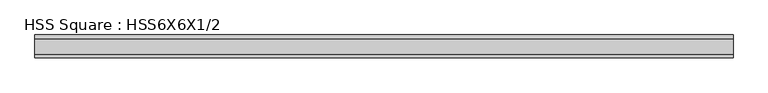
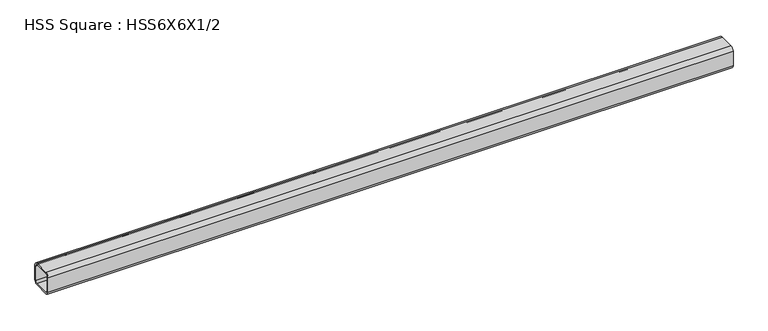
"""IFC4 building model written with IfcOpenShell, lengths in millimetres: member geometry, HSS Square : HSS6X6X1/2."""

from ifc_helpers import new_model, si_unit, point, frame, frame_2d, origin, place, context, project, spatial, polyline, circle_curve, trimmed, segment, composite_curve, outline, extrude, source, transform, mapped, element, save


def hss_square_hss6x6x1_2_53b34d95(model_context):
    return source(origin(), model_context, "Body", "SweptSolid", [
        extrude(outline(composite_curve([segment(polyline([(76.2, 50.8), (76.2, -50.8)]), True, "CONTINUOUS"), segment(trimmed(circle_curve(frame_2d((50.8, -50.8)), 25.4), [point((76.2, -50.8))], [point((50.8, -76.2))], False, "CARTESIAN"), True, "CONTINUOUS"), segment(polyline([(50.8, -76.2), (-50.8, -76.2)]), True, "CONTINUOUS"), segment(trimmed(circle_curve(frame_2d((-50.8, -50.8)), 25.4), [point((-50.8, -76.2))], [point((-76.2, -50.8))], False, "CARTESIAN"), True, "CONTINUOUS"), segment(polyline([(-76.2, -50.8), (-76.2, 50.8)]), True, "CONTINUOUS"), segment(trimmed(circle_curve(frame_2d((-50.8, 50.8)), 25.4), [point((-76.2, 50.8))], [point((-50.8, 76.2))], False, "CARTESIAN"), True, "CONTINUOUS"), segment(polyline([(-50.8, 76.2), (50.8, 76.2)]), True, "CONTINUOUS"), segment(trimmed(circle_curve(frame_2d((50.8, 50.8)), 25.4), [point((50.8, 76.2))], [point((76.2, 50.8))], False, "CARTESIAN"), True, "CONTINUOUS")], self_intersect=False), holes=[composite_curve([segment(trimmed(circle_curve(frame_2d((-50.8, 50.8)), 12.7), [point((-50.8, 63.5))], [point((-63.5, 50.8))], True, "CARTESIAN"), True, "CONTINUOUS"), segment(polyline([(-63.5, 50.8), (-63.5, -50.8)]), True, "CONTINUOUS"), segment(trimmed(circle_curve(frame_2d((-50.8, -50.8)), 12.7), [point((-63.5, -50.8))], [point((-50.8, -63.5))], True, "CARTESIAN"), True, "CONTINUOUS"), segment(polyline([(-50.8, -63.5), (50.8, -63.5)]), True, "CONTINUOUS"), segment(trimmed(circle_curve(frame_2d((50.8, -50.8)), 12.7), [point((50.8, -63.5))], [point((63.5, -50.8))], True, "CARTESIAN"), True, "CONTINUOUS"), segment(polyline([(63.5, -50.8), (63.5, 50.8)]), True, "CONTINUOUS"), segment(trimmed(circle_curve(frame_2d((50.8, 50.8)), 12.7), [point((63.5, 50.8))], [point((50.8, 63.5))], True, "CARTESIAN"), True, "CONTINUOUS"), segment(polyline([(50.8, 63.5), (-50.8, 63.5)]), True, "CONTINUOUS")], self_intersect=False)]), frame((-2344.7522436, 0.0, 0.0), z_axis=(1.0, 0.0, 0.0), x_axis=(0.0, 1.0, 0.0)), (0.0, 0.0, 1.0), 4615.1338001),
    ])


if __name__ == "__main__":
    model = new_model("IFC4")
    model_context = context("Model", 3, world=origin())
    ifc_project = project(units=[si_unit("LENGTHUNIT", "METRE", prefix="MILLI")], contexts=[model_context])
    site = spatial("IfcSite", under=ifc_project)
    building = spatial("IfcBuilding", under=site)
    placement = place(None, origin())
    hss_square_hss6x6x1_2_shape = hss_square_hss6x6x1_2_53b34d95(model_context)
    element("IfcMember", 1, ObjectType="HSS Square : HSS6X6X1/2", at=placement, inside=building, context=model_context, shape_type="MappedRepresentation", body=[
        mapped(hss_square_hss6x6x1_2_shape, transform((0.0, 0.0, 0.0), x_axis=(1.0, 0.0, 0.0), y_axis=(0.0, 1.0, 0.0), z_axis=(0.0, 0.0, 1.0))),
    ])
    save(model, "model.ifc")

# Revit data of these elements
# Type "HSS Square : HSS6X6X1/2"
#   Section Name Key = "HSS 6X6X1/2"
#   Assembly Code = "B10"
#   Width = 6.000"
#   Wall Nominal Thickness = 0.500"
#   Wall Design Thickness = 0.465"
#   Torsional Moment of Inertia = 81.10 in⁴
#   Torsional Modulus = 28.10 in³
#   Section Area = 9.74 in²
#   Plastic Modulus weak axis = 19.80 in³
#   Plastic Modulus strong axis = 19.80 in³
#   Outer Fillet = 1.000"
#   Nominal Weight = 35.24 lbf/ft
#   Moment of Inertia weak axis = 48.30 in⁴
#   Moment of Inertia strong axis = 48.30 in⁴
#   Inner Fillet = 0.500"
#   Height = 6.000"
#   Elastic Modulus weak axis = 16.10 in³
#   Elastic Modulus strong axis = 16.10 in³
#   Centroid Vertical = 3.000"
#   Centroid Horizontal = 3.000"
#   Length [instance default] = 5' - 0"
#   Structural Material [instance default] = Steel ASTM A500, Grade B, Rectangular and Square
#   Principal Axes Angle = 0
# Element 1 (IfcMember, "HSS Square : HSS6X6X1/2")
#   Structural Material = Steel ASTM A992
#   Materials on its faces: "Steel ASTM A992"
# Materials
#   "Steel ASTM A500, Grade B, Rectangular and Square": class "Metal", colour RGB 199 199 199, transparency 0, Description = "Carbon steel", Cost = 0
#   "Steel ASTM A992": class "Metal", colour RGB 199 199 199, transparency 0, Description = "Structural steel 50ksi", Cost = 0
